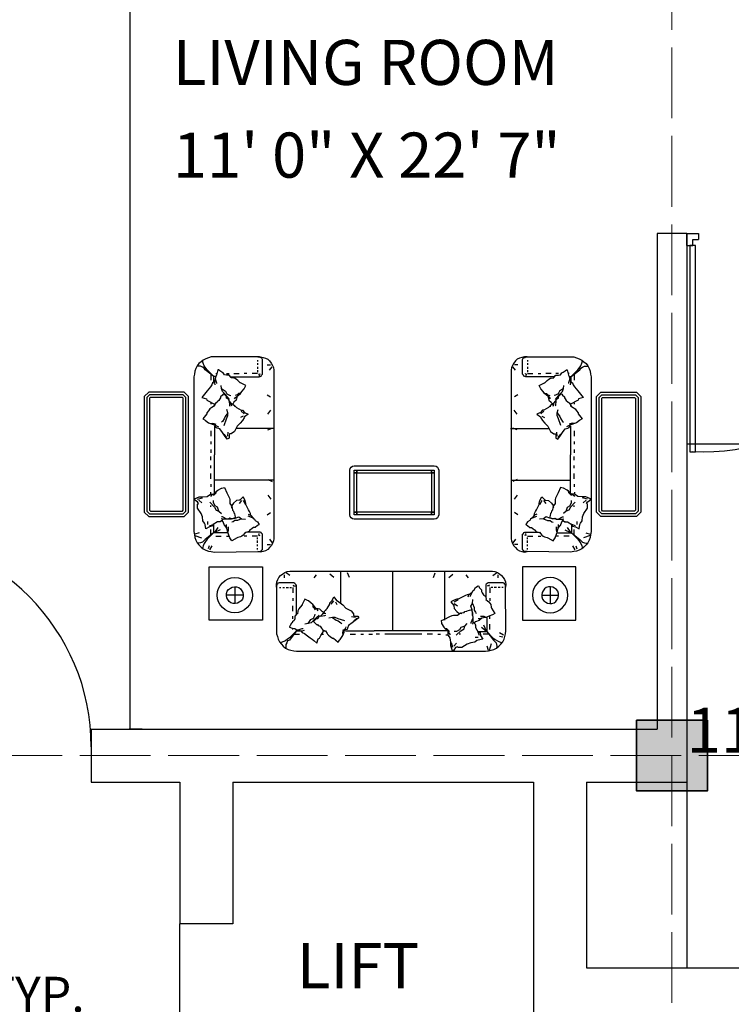
# Model space of a CAD drawing. Units: inches. Extents: x -113 to 5399, y -1393 to 3302.
# Tile 7 of 40: x 1073 to 1194, y 460 to 627. Entities that reach past the tile are written whole.
import ezdxf

# ---------------------------------------------------------------- set-up
doc = ezdxf.new("R2010")
doc.units = ezdxf.units.IN
doc.header["$MEASUREMENT"] = 0
doc.linetypes.add('ACAD_ISO02W100', pattern=[15, 12, -3])
doc.layers.add('24', color=7, linetype='Continuous')
for name, color, linetype, lineweight in [('A-ANNO-DIMS', 254, 'Continuous', 18), ('A-AREA-IDEN', 4, 'Continuous', 18), ('A-COLS', 7, 'Continuous', 35), ('doors', 2, 'Continuous', 25), ('furniture', 131, 'Continuous', 18), ('GRIDS', 7, 'ACAD_ISO02W100', 13), ('walls', 1, 'Continuous', 25)]:
    doc.layers.add(name, color=color, linetype=linetype, lineweight=lineweight)
doc.styles.get("Standard").update_dxf_attribs({"font": 'arial.ttf'})
doc.dimstyles.get("Standard").update_dxf_attribs({"dimtxt": 6, "dimasz": 0.18, "dimexe": 0.18, "dimexo": 0.0625, "dimgap": 0.09, "dimtad": 0, "dimtih": 1, "dimtoh": 1, "dimdec": 1, "dimzin": 0, "dimdsep": 46, "dimlunit": 4, "dimtxsty": 'Standard', "dimblk": 'ARCHTICK', "dimcen": 0.09, "dimadec": 0, "dimazin": 0, "dimtfac": 1, "dimtdec": 1, "dimtofl": 0, "dimtmove": 0, "dimatfit": 3, "dimfxl": 1, "dimtolj": 1, "dimtzin": 0, "dimarcsym": 0})

# ---------------------------------------------------------------- blocks, each defined once
blk = doc.blocks.new('*U3')
for p, q in [((0, 0), (0, -6)), ((36, 0), (36, -6))]:
    blk.add_line(p, q)
blk.add_lwpolyline([(0, 0), (0, 36), (1.75, 36), (1.75, 0)], close=True)
blk.add_arc((0, 0), 36, 0, 90)
blk = doc.blocks.new('DL13712')
at = {"layer": '24'}
for p, q in [((33, 28.5), (-34, 28.5)), ((33.5, -29.5), (-10, -29.5))]:
    blk.add_line(p, q, dxfattribs=at)
blk = doc.blocks.new('DL13976')
at = {"layer": '24'}
for p, q in [((-16, 11), (-13.5, 14)), ((-13.5, 14), (-10.5, 16.5)), ((-10.5, 16.5), (-7, 18.5)), ((-7, 18.5), (-3.5, 19.5)), ((-3.5, 19.5), (0.5, 20)), ((0.5, 20), (4.5, 19.5)), ((4.5, 19.5), (8, 18.5)), ((8, 18.5), (11.5, 16.5)), ((11.5, 16.5), (14.5, 14)), ((14.5, 14), (17, 11)), ((-19.5, 0), (-19, 4)), ((-19, -4), (-19.5, 0)), ((-19, 4), (-18, 7.5)), ((-18, 7.5), (-16, 11)), ((-9, 2), (-8, 4.5)), ((-9, -0.5), (-9, 2)), ((-9, 0), (10, 0)), ((-8, 4.5), (-6.5, 6.5)), ((-6.5, 6.5), (-4.5, 8)), ((-5.5, 0), (6.5, 0)), ((-4.5, 8), (-2.5, 9)), ((-2.5, 9), (0, 9.5)), ((0, 9.5), (2.5, 9.5)), ((0.5, -9.5), (0.5, 9.5)), ((0.5, -6), (0.5, 6)), ((2.5, 9.5), (5, 8.5)), ((5, 8.5), (7, 7)), ((7, 7), (8.5, 5)), ((8.5, 5), (9.5, 3)), ((9.5, 3), (10, 0.5)), ((10, 0.5), (10, -2)), ((17, 11), (19, 7.5)), ((19, 7.5), (20, 4)), ((20, 4), (20.5, 0)), ((20.5, 0), (20, -4)), ((-18, -7.5), (-19, -4)), ((-16, -11), (-18, -7.5)), ((-13.5, -14), (-16, -11)), ((-8.5, -3), (-9, -0.5)), ((-7.5, -5), (-8.5, -3)), ((-6, -7), (-7.5, -5)), ((-4, -8.5), (-6, -7)), ((-1.5, -9.5), (-4, -8.5)), ((1, -9.5), (-1.5, -9.5)), ((3.5, -9), (1, -9.5)), ((5.5, -8), (3.5, -9)), ((7.5, -6.5), (5.5, -8)), ((9, -4.5), (7.5, -6.5)), ((10, -2), (9, -4.5)), ((17, -11), (14.5, -14)), ((19, -7.5), (17, -11)), ((20, -4), (19, -7.5)), ((-10.5, -16.5), (-13.5, -14)), ((-7, -18.5), (-10.5, -16.5)), ((-3.5, -19.5), (-7, -18.5)), ((0.5, -20), (-3.5, -19.5)), ((4.5, -19.5), (0.5, -20)), ((8, -18.5), (4.5, -19.5)), ((11.5, -16.5), (8, -18.5)), ((14.5, -14), (11.5, -16.5))]:
    blk.add_line(p, q, dxfattribs=at)
blk = doc.blocks.new('DL13329')
at = {"layer": '24'}
for p, q in [((0, 0), (0, -60)), ((60, 0), (0, 0)), ((60, -60), (60, 0)), ((0, -60), (60, -60))]:
    blk.add_line(p, q, dxfattribs=at)
blk = doc.blocks.new('DL13303')
at = {"layer": '24'}
for p, q in [((-70, 20), (-65, 25)), ((-65, 25), (65, 25)), ((65, 25), (70, 20)), ((-70, -20), (-70, 20)), ((-67, 19), (-64, 22)), ((-67, -19), (-67, 19)), ((-64, 22), (64, 22)), ((-64, 18), (-63, 19)), ((-64, -18), (-64, 18)), ((-63, 19), (63, 19)), ((63, 19), (64, 18)), ((64, 22), (67, 19)), ((64, 18), (64, -18)), ((67, 19), (67, -19)), ((70, 20), (70, -20)), ((-65, -25), (-70, -20)), ((-64, -22), (-67, -19)), ((-63, -19), (-64, -18)), ((64, -22), (-64, -22)), ((63, -19), (-63, -19)), ((64, -18), (63, -19)), ((67, -19), (64, -22)), ((70, -20), (65, -25)), ((65, -25), (-65, -25))]:
    blk.add_line(p, q, dxfattribs=at)
blk = doc.blocks.new('DL12701')
at = {"layer": '24'}
for p, q in [((-96.5, 43.5), (-93.5, 44.5)), ((-93.5, 44.5), (-90, 45)), ((-90, 45), (-87, 45.5)), ((-87, 45.5), (0, 45.5)), ((0, 45.5), (87, 45.5)), ((50, 45), (48, 39.5)), ((51.5, 44.5), (50, 45)), ((53.5, 41.5), (51.5, 44.5)), ((87, 45.5), (90.5, 45)), ((88.5, 39.5), (90, 44.5)), ((90.5, 45), (93.5, 44.5)), ((91.5, 44.5), (94, 37)), ((93.5, 44.5), (96.5, 43.5)), ((-107.5, 32), (-106, 35)), ((-106, 35), (-104, 37.5)), ((-102.5, 35), (-105, 36)), ((-104, 37.5), (-102, 40)), ((-99.5, 34), (-102.5, 35)), ((-102, 40), (-99.5, 42)), ((-99.5, 42), (-96.5, 43.5)), ((-97, 32), (-99.5, 34)), ((-99, 40), (-99, 42)), ((-99, 38), (-99, 40)), ((-98, 36), (-99, 38)), ((-97, 34), (-98, 36)), ((-95, 33), (-97, 34)), ((-69.5, 32), (-67.5, 33.5)), ((-67.5, 33.5), (-64, 36.5)), ((-64, 36.5), (-62.5, 31.5)), ((-45.5, 31), (-40, 35.5)), ((-40, 35.5), (-38.5, 33)), ((48, 35.5), (47.5, 30.5)), ((48, 39.5), (48, 35.5)), ((50.5, 41.5), (49, 36)), ((51.5, 40), (54.5, 36.5)), ((55.5, 40.5), (53.5, 41.5)), ((56, 41.5), (55.5, 40.5)), ((60.5, 41.5), (56, 41.5)), ((66.5, 37.5), (60.5, 41.5)), ((70.5, 36), (66.5, 37.5)), ((75, 35.5), (70.5, 36)), ((77.5, 33.5), (75, 35.5)), ((79, 33), (77.5, 33.5)), ((96, 33), (97.5, 34.5)), ((96.5, 43.5), (99.5, 42)), ((97.5, 34.5), (99, 36)), ((98, 32.5), (100.5, 34)), ((99, 36), (99.5, 38)), ((99.5, 42), (102, 40)), ((100, 40), (99.5, 42)), ((99.5, 38), (100, 40)), ((100.5, 34), (103, 35)), ((102, 40), (104.5, 37.5)), ((103, 35), (106, 36)), ((104.5, 37.5), (106.5, 35)), ((106.5, 35), (108, 32)), ((-109.5, 26), (-108.5, 29)), ((-109.5, 22.5), (-109.5, 26)), ((-109.5, -26.5), (-109.5, 22.5)), ((-108.5, 29), (-107.5, 32)), ((-95, 30.5), (-97, 32)), ((-87.5, 23), (-95, 33)), ((-87.5, 23), (-95, 30.5)), ((-89.5, 26.5), (-83.5, 26.5)), ((-87.5, 21), (-87.5, 23)), ((-81.5, 23), (-87.5, 23)), ((-85, 21.5), (-82, 22.5)), ((-82, 22.5), (-80.5, 24.5)), ((-82, 22.5), (-80.5, 22.5)), ((-80.5, 24.5), (-78, 25.5)), ((-80.5, 24.5), (-80.5, 23.5)), ((-80.5, 22.5), (-78, 22)), ((-78, 25.5), (-76, 27)), ((-77, 25.5), (-77, 25.5)), ((-76, 27), (-71.5, 30.5)), ((-71.5, 30.5), (-69.5, 32)), ((-62.5, 31.5), (-61, 31)), ((-61, 31), (-59.5, 28)), ((-59.5, 28), (-57.5, 24.5)), ((-58, 26.5), (-56.5, 26.5)), ((-58, 21), (-54.5, 23)), ((-57.5, 24.5), (-56.5, 22)), ((-56.5, 22.5), (-54.5, 22.5)), ((-54.5, 22.5), (-52.5, 25.5)), ((-54.5, 23), (-54.5, 22.5)), ((-54, 22.5), (-54, 22.5)), ((-52.5, 25.5), (-52, 26.5)), ((-52, 26.5), (-51, 27.5)), ((-51, 27.5), (-49, 29)), ((-49, 29), (-46.5, 31)), ((-46.5, 31), (-45.5, 31)), ((-38.5, 33), (-38, 32.5)), ((-38, 32.5), (-35.5, 29)), ((-35.5, 29), (-34.5, 27)), ((-34.5, 27), (-35, 24.5)), ((-35, 24.5), (-34.5, 23)), ((-34.5, 27), (-33.5, 24)), ((-34.5, 23), (-34, 21)), ((-33.5, 24), (-33, 22)), ((-32, 22.5), (0.5, 22.5)), ((-26.5, 26.5), (-20.5, 26.5)), ((-14.5, 26.5), (-11.5, 26.5)), ((-5.5, 26.5), (-1.5, 26.5)), ((44, 22.5), (0.5, 22.5)), ((6.5, 26.5), (2.5, 26.5)), ((15.5, 26.5), (12.5, 26.5)), ((27.5, 26.5), (21.5, 26.5)), ((33.5, 26.5), (36.5, 26.5)), ((42.5, 27), (45, 27)), ((45, 23.5), (43.5, 22)), ((45.5, 28), (45, 27)), ((45, 27), (45, 23.5)), ((45, 23.5), (46.5, 26)), ((46.5, 23.5), (45, 22)), ((47.5, 30.5), (45.5, 28)), ((46.5, 26), (47.5, 27)), ((54.5, 23.5), (52, 23.5)), ((54, 27.5), (59.5, 22.5)), ((58, 21.5), (54.5, 23.5)), ((59, 26.5), (57.5, 26.5)), ((59.5, 22.5), (63, 20.5)), ((79, 30), (75.5, 30)), ((76, 19), (79, 24)), ((84, 32), (79, 33)), ((80.5, 28), (79, 24)), ((79, 24), (81, 24.5)), ((79, 23.5), (88.5, 23.5)), ((81, 24.5), (81.5, 28)), ((81.5, 28), (84, 32)), ((82.5, 18.5), (88, 22.5)), ((90.5, 26.5), (84.5, 26.5)), ((85, 16), (88, 22.5)), ((88.5, 23.5), (96, 33)), ((88.5, 23.5), (95.5, 30.5)), ((88.5, 8), (88.5, 23.5)), ((95.5, 30.5), (98, 32.5)), ((103, 28.5), (106.5, 29.5)), ((107.5, 27.5), (103, 25)), ((108, 32), (109, 29)), ((109, 29), (109.5, 26)), ((109.5, 26), (110, 22.5)), ((110, 22.5), (109.5, -26.5)), ((-95, 18.5), (-92, 19.5)), ((-95, 18), (-95, 18.5)), ((-94, 16.5), (-95, 18)), ((-92.5, 14), (-94, 16.5)), ((-92, 13.5), (-92.5, 14)), ((-92, 19.5), (-89, 20)), ((-91.5, 12.5), (-92, 13.5)), ((-89.5, 11), (-91.5, 12.5)), ((-91, 21), (-91, 19.5)), ((-89, 20), (-87.5, 21)), ((-87.5, 21), (-85, 21.5)), ((-85, 21.5), (-80.5, 20)), ((-80.5, 20), (-79.5, 20)), ((-74, 14.5), (-77.5, 15)), ((-70.5, 13.5), (-74, 14.5)), ((-74, 14.5), (-71, 10)), ((-67.5, 10.5), (-70.5, 13.5)), ((-68, 12), (-67.5, 12.5)), ((-65, 9), (-68, 12)), ((-67.5, 12.5), (-66.5, 13.5)), ((-66.5, 13.5), (-64.5, 15.5)), ((-64.5, 15.5), (-63.5, 15.5)), ((-63.5, 15.5), (-62.5, 16.5)), ((-62.5, 16.5), (-60.5, 17.5)), ((-60.5, 17.5), (-59, 19.5)), ((-59, 19.5), (-58.5, 19.5)), ((-58.5, 19.5), (-58, 21)), ((-42.5, 10.5), (-40, 11.5)), ((-40, 11.5), (-37, 13.5)), ((-32.5, 11.5), (-40, 9)), ((-37, 13.5), (-36, 14.5)), ((-30, 21), (-33, 22)), ((-33, 22), (-31.5, 19.5)), ((-31.5, 19.5), (-31, 18)), ((-29.5, 19.5), (-30, 21)), ((-28.5, 16.5), (-29.5, 19.5)), ((-24.5, 13.5), (-28.5, 16.5)), ((-21, 11), (-24.5, 13.5)), ((-19, 8.5), (-22.5, 11.5)), ((38, 14), (37.5, 11)), ((40.5, 18.5), (38, 14.5)), ((38, 14.5), (38, 14)), ((41.5, 20), (40.5, 18.5)), ((43.5, 22), (41.5, 20)), ((43.5, 20.5), (41.5, 20)), ((45, 22), (43.5, 20.5)), ((59.5, 19), (58, 21.5)), ((64, 17.5), (59.5, 19)), ((63, 20.5), (64, 17.5)), ((64, 17.5), (66.5, 14.5)), ((70.5, 13.5), (70.5, 14.5)), ((73, 8.5), (70.5, 13.5)), ((73, 13), (72.5, 15)), ((73, 12.5), (75, 14.5)), ((73, 12.5), (73, 13)), ((73, 8.5), (73, 12.5)), ((76, 12.5), (74, 14)), ((75, 14.5), (76, 16)), ((75.5, 16), (76, 16.5)), ((76, 16), (76, 19)), ((80, 11), (76, 12.5)), ((92, 21), (92, 15)), ((-91, 9), (-91, 6)), ((-91, 0.5), (-91, -5.5)), ((-89, 9), (-89.5, 11)), ((-89, 8.5), (-89, 9)), ((-89, 6), (-89, 8.5)), ((-86.5, 3.5), (-89, 6)), ((-87, 3.5), (-87, -26.5)), ((-86, 3.5), (-86.5, 3.5)), ((-85.5, 0.5), (-86, 3.5)), ((-85.5, 0), (-85.5, 0.5)), ((-84.5, -2), (-85.5, 0)), ((-71, 10), (-68, 8.5)), ((-68, 8.5), (-66.5, 5.5)), ((-61.5, 5.5), (-67.5, 10.5)), ((-66.5, 5.5), (-66, 4)), ((-63, 9), (-65, 9)), ((-62.5, 0), (-63.5, -1)), ((-62, 6.5), (-63, 9)), ((-60, 6), (-62, 6.5)), ((-61, -2), (-58.5, 0.5)), ((-57.5, 3.5), (-60, 6)), ((-60, 6), (-55, 5.5)), ((-58.5, 0.5), (-55.5, 2)), ((-56.5, 3.5), (-57.5, 3.5)), ((-57.5, 3.5), (-56, 1.5)), ((-54, 3), (-56.5, 3.5)), ((-56, 1.5), (-55, 0)), ((-55, 5.5), (-54, 5)), ((-55, 0), (-52.5, -2.5)), ((-46.5, 7.5), (-50.5, 8.5)), ((-46.5, 7.5), (-42.5, 10.5)), ((-43.5, 7.5), (-46.5, 7.5)), ((-40, 9), (-43.5, 7.5)), ((-31.5, -3), (-25.5, 0)), ((-25.5, 0), (-23, 3.5)), ((-20.5, 7.5), (-25, 7)), ((-23, 5.5), (-21.5, 6)), ((-23, 3.5), (-23, 5.5)), ((-21.5, 6), (-18, 6)), ((-17, 8), (-21, 11)), ((-18, 6), (-17, 8)), ((37.5, 11), (43.5, 8.5)), ((43.5, 8.5), (44, 8)), ((44, 8), (47, 6.5)), ((47, 6.5), (49.5, 5.5)), ((49.5, 5.5), (51, 5)), ((51, 5), (52.5, 5)), ((52, -2.5), (55, 1)), ((52.5, 5), (55.5, 5)), ((55, 1), (57.5, 3)), ((55.5, 5), (55.5, 5)), ((55.5, 5), (59, 2.5)), ((59, 2.5), (60, 3.5)), ((60, 3.5), (60, 2.5)), ((60, 2.5), (63, 2)), ((63, 2), (64, 1)), ((64, 1), (66, 0.5)), ((66, 0.5), (66.5, 0)), ((66.5, 0), (69, -0.5)), ((71.5, -1), (72.5, 2.5)), ((72, 5), (73, 6.5)), ((73, 5.5), (72, -1)), ((72.5, 2.5), (72, 5)), ((73, 6.5), (73, 8.5)), ((74.5, -0.5), (76, 1.5)), ((76, 1.5), (76.5, 3)), ((80.5, 9), (79, 9)), ((80.5, 10.5), (80, 11)), ((83, 8.5), (80.5, 10.5)), ((83, 8.5), (80.5, 9)), ((84, 6.5), (81.5, 6.5)), ((85, 8), (83, 8.5)), ((85.5, 6.5), (84, 6.5)), ((88, 7.5), (85, 8)), ((88, 7.5), (85.5, 6.5)), ((90, 6.5), (88, 7.5)), ((94, 5), (90, 6.5)), ((92, 9), (92, 6)), ((95, 4.5), (94, 5)), ((94, -3), (97.5, 3)), ((97.5, 3), (95, 4.5)), ((-91, -14), (-91, -11)), ((-83, -4), (-84.5, -2)), ((-80.5, -6.5), (-83, -4)), ((-80.5, -7), (-80.5, -6.5)), ((-77.5, -13), (-80.5, -7)), ((-73.5, -11), (-74.5, -11.5)), ((-70.5, -8.5), (-73.5, -11)), ((-68.5, -7), (-70.5, -8.5)), ((-68.5, -4.5), (-67, -3)), ((-66.5, -4.5), (-68.5, -7)), ((-68.5, -7), (-68.5, -4.5)), ((-67, -3), (-66, -1)), ((-65.5, -3), (-66.5, -4.5)), ((-63.5, -1), (-65.5, -3)), ((-65.5, -3), (-62.5, -2.5)), ((-62.5, -2.5), (-61, -2)), ((-54, -0.5), (-53.5, -0.5)), ((-52.5, -2.5), (-49.5, -7.5)), ((-49.5, -7.5), (-49.5, -9)), ((-49.5, -9), (-47, -11.5)), ((-45.5, -11), (-48.5, -7.5)), ((-43, -10), (-41.5, -7)), ((-42, -11.5), (-41, -11)), ((-41, -11), (-38, -9)), ((-38, -9), (-35, -6.5)), ((-35, -6.5), (-31.5, -3)), ((48, -10), (51.5, -6)), ((52, -12), (48, -10)), ((51.5, -5.5), (52, -2.5)), ((51.5, -6), (51.5, -5.5)), ((52, -8), (55.5, -5.5)), ((52, -10), (56.5, -12.5)), ((69, -0.5), (70.5, -1)), ((70.5, -1), (71.5, -1)), ((72, -1), (70.5, -5)), ((70.5, -5), (72.5, -8)), ((72.5, -8), (74.5, -3.5)), ((72.5, -8), (73, -12.5)), ((74.5, -3.5), (74.5, -0.5)), ((87.5, -12.5), (89.5, -11)), ((89.5, -11), (91, -10)), ((91, -10), (92, -8.5)), ((92, -8.5), (93, -7)), ((92, -14), (92, -11)), ((93, -7), (93.5, -4)), ((93.5, -4), (94, -3)), ((-91, -26), (-91, -20)), ((-74.5, -11.5), (-77.5, -13)), ((-47, -11.5), (-45, -15.5)), ((-45, -15.5), (-42, -11.5)), ((55, -13), (52, -12)), ((56.5, -13), (55, -13)), ((62.5, -16), (56.5, -13)), ((64.5, -17), (62.5, -16)), ((64, -16.5), (64, -16.5)), ((66.5, -18), (64.5, -17)), ((69, -18.5), (66.5, -18)), ((67.5, -15.5), (68.5, -18)), ((68.5, -18), (69, -18.5)), ((69, -18.5), (72, -21)), ((70, -16.5), (69.5, -15.5)), ((72, -21), (70, -16.5)), ((72, -21), (73, -22.5)), ((82.5, -21.5), (83.5, -20)), ((82.5, -22.5), (82.5, -21.5)), ((83.5, -20), (85, -18)), ((85, -17.5), (87, -16.5)), ((85, -18), (85, -17.5)), ((87, -16.5), (88, -13)), ((88, -13), (87.5, -12.5)), ((87.5, -26.5), (87.5, -14.5)), ((92, -26), (92, -20)), ((-109.5, -28), (-109.5, -26.5)), ((-109.5, -26.5), (-109.5, -29.5)), ((-109, -29), (-109.5, -28)), ((-109.5, -29.5), (-109, -32.5)), ((-108.5, -30), (-109, -29)), ((-109, -32.5), (-108, -35)), ((-108, -31), (-108.5, -30)), ((-106.5, -31.5), (-108, -31)), ((-105.5, -31.5), (-106.5, -31.5)), ((-106, -26), (-104.5, -26)), ((-104.5, -31.5), (-105.5, -31.5)), ((-92, -31.5), (-104.5, -31.5)), ((-102.5, -26), (-100.5, -26)), ((-98.5, -26), (-96, -26)), ((-94.5, -26), (-92.5, -26)), ((-91, -31.5), (-92, -31.5)), ((-90, -31.5), (-91, -31.5)), ((-90.5, -27.5), (-88, -28)), ((-90.5, -28), (-90, -29)), ((-89, -30.5), (-90, -31.5)), ((-88, -30), (-89, -30.5)), ((-87.5, -29), (-88, -30)), ((-87, -28), (-87.5, -29)), ((-87, -26.5), (-87, -28)), ((73, -22.5), (74.5, -23.5)), ((74.5, -23.5), (76, -26)), ((76, -26), (79, -28)), ((79, -28), (79.5, -27.5)), ((79.5, -27.5), (80, -26)), ((80, -26), (82.5, -23.5)), ((82.5, -23.5), (82.5, -22.5)), ((87.5, -28), (87.5, -26.5)), ((87.5, -29), (87.5, -28)), ((88, -30), (87.5, -29)), ((89, -30.5), (88, -30)), ((91.5, -27.5), (89, -28)), ((90, -31.5), (89, -30.5)), ((91, -31.5), (90, -31.5)), ((91.5, -28), (91, -29)), ((92.5, -31.5), (91, -31.5)), ((104.5, -31.5), (92.5, -31.5)), ((95.5, -26), (93.5, -26)), ((99.5, -26), (97, -26)), ((103.5, -26), (101.5, -26)), ((106, -31.5), (104.5, -31.5)), ((107, -26), (105.5, -26)), ((107, -31.5), (106, -31.5)), ((108, -31), (107, -31.5)), ((109, -30), (108, -31)), ((108.5, -35), (109.5, -32.5)), ((109.5, -29), (109, -30)), ((110, -29.5), (109.5, -26.5)), ((109.5, -26.5), (109.5, -28)), ((109.5, -28), (109.5, -29)), ((109.5, -32.5), (110, -29.5)), ((-108, -35), (-107, -37.5)), ((-107, -37.5), (-105, -39.5)), ((-105, -39.5), (-102.5, -41.5)), ((-102.5, -41.5), (-100, -43)), ((-100.5, -37), (-100.5, -40.5)), ((-100, -43), (-97.5, -44)), ((-94.5, -39.5), (-98.5, -42.5)), ((-97.5, -44), (-94.5, -44.5)), ((-67, -37), (-64.5, -40.5)), ((-45, -37.5), (-49.5, -41)), ((-27.5, -37.5), (-29.5, -42.5)), ((28.5, -37.5), (30.5, -42.5)), ((46, -37.5), (50.5, -41)), ((68, -37), (65.5, -40.5)), ((95, -44.5), (97.5, -44)), ((95.5, -39.5), (99.5, -42.5)), ((97.5, -44), (100.5, -43)), ((100.5, -43), (103, -41.5)), ((101.5, -37), (101.5, -40.5)), ((103, -41.5), (105, -39.5)), ((105, -39.5), (107, -37.5)), ((107, -37.5), (108.5, -35)), ((-94.5, -44.5), (0, -44.5)), ((0, -44.5), (95, -44.5))]:
    blk.add_line(p, q, dxfattribs=at)
blk = doc.blocks.new('DL13707')
at = {"layer": '24'}
for p, q in [((0, -33.5), (0, 33.5)), ((-58.5, -33.5), (-58.5, 21.5)), ((58.5, -33.5), (58.5, 2))]:
    blk.add_line(p, q, dxfattribs=at)
blk = doc.blocks.new('DL13651')
at = {"layer": '24'}
for p, q in [((-50.5, 25), (-50, 27)), ((-50.5, -25), (-50.5, 25)), ((-50, 27), (-49, 28.5)), ((-49, 28.5), (-47.5, 29.5)), ((-47.5, 29.5), (-45.5, 30)), ((-45.5, 30), (44.5, 30)), ((-45.5, 24.5), (-45.5, 25)), ((-45.5, 25), (-45, 25)), ((-45.5, -24.5), (-45.5, 24.5)), ((-45, 25), (44, 25)), ((-42.5, -24.5), (-42.5, 24.5)), ((-42.5, 24.5), (-42.5, 22)), ((41.5, 22), (41.5, 24.5)), ((41.5, 24.5), (41.5, -24.5)), ((44, 25), (44.5, 25)), ((44.5, 30), (46.5, 29.5)), ((44.5, 25), (44.5, 24.5)), ((44.5, 24.5), (44.5, -24.5)), ((46.5, 29.5), (48, 28.5)), ((48, 28.5), (49, 27)), ((49, 27), (49.5, 25)), ((49.5, 25), (49.5, -25)), ((-45, 22), (44, 22)), ((-42.5, 22), (-45, 22)), ((44, 22), (41.5, 22)), ((44, -22), (-45, -22)), ((-45, -22), (-42.5, -22)), ((-42.5, -22), (-42.5, -24.5)), ((41.5, -24.5), (41.5, -22)), ((41.5, -22), (44, -22)), ((-50, -27), (-50.5, -25)), ((-49, -28.5), (-50, -27)), ((-47.5, -29.5), (-49, -28.5)), ((-45.5, -30), (-47.5, -29.5)), ((-45.5, -25), (-45.5, -24.5)), ((-45, -25), (-45.5, -25)), ((44.5, -30), (-45.5, -30)), ((44, -25), (-45, -25)), ((44.5, -25), (44, -25)), ((44.5, -24.5), (44.5, -25)), ((46.5, -29.5), (44.5, -30)), ((48, -28.5), (46.5, -29.5)), ((49, -27), (48, -28.5)), ((49.5, -25), (49, -27))]:
    blk.add_line(p, q, dxfattribs=at)
blk = doc.blocks.new('DL12263')
at = {"layer": '24'}
for p, q in [((-115.5, 43.5), (-112.5, 44.5)), ((-112.5, 44.5), (-109, 45)), ((-109, 45), (-106, 45.5)), ((-106, 45.5), (-19, 45.5)), ((-19, 45.5), (106.5, 45.5)), ((69.5, 45), (67.5, 39.5)), ((71, 44.5), (69.5, 45)), ((73, 41.5), (71, 44.5)), ((106.5, 45.5), (110, 45)), ((108, 39.5), (109.5, 44.5)), ((110, 45), (113, 44.5)), ((111, 44.5), (113.5, 37)), ((113, 44.5), (116, 43.5)), ((-126.5, 32), (-125, 35)), ((-125, 35), (-123, 37.5)), ((-121.5, 35), (-124, 36)), ((-123, 37.5), (-121, 40)), ((-118.5, 34), (-121.5, 35)), ((-121, 40), (-118.5, 42)), ((-118.5, 42), (-115.5, 43.5)), ((-116, 32), (-118.5, 34)), ((-118, 40), (-118, 42)), ((-118, 38), (-118, 40)), ((-117, 36), (-118, 38)), ((-116, 34), (-117, 36)), ((-114, 33), (-116, 34)), ((-88.5, 32), (-86.5, 33.5)), ((-86.5, 33.5), (-83, 36.5)), ((-83, 36.5), (-81.5, 31.5)), ((-64.5, 31), (-59, 35.5)), ((-59, 35.5), (-57.5, 33)), ((67.5, 35.5), (67, 30.5)), ((67.5, 39.5), (67.5, 35.5)), ((70, 41.5), (68.5, 36)), ((71, 40), (74, 36.5)), ((75, 40.5), (73, 41.5)), ((75.5, 41.5), (75, 40.5)), ((80, 41.5), (75.5, 41.5)), ((86, 37.5), (80, 41.5)), ((90, 36), (86, 37.5)), ((94.5, 35.5), (90, 36)), ((97, 33.5), (94.5, 35.5)), ((98.5, 33), (97, 33.5)), ((115.5, 33), (117, 34.5)), ((116, 43.5), (119, 42)), ((117, 34.5), (118.5, 36)), ((117.5, 32.5), (120, 34)), ((118.5, 36), (119, 38)), ((119, 42), (121.5, 40)), ((119.5, 40), (119, 42)), ((119, 38), (119.5, 40)), ((120, 34), (122.5, 35)), ((121.5, 40), (124, 37.5)), ((122.5, 35), (125.5, 36)), ((124, 37.5), (126, 35)), ((126, 35), (127.5, 32)), ((-128.5, 26), (-127.5, 29)), ((-128.5, 22.5), (-128.5, 26)), ((-128.5, -26.5), (-128.5, 22.5)), ((-127.5, 29), (-126.5, 32)), ((-114, 30.5), (-116, 32)), ((-106.5, 23), (-114, 33)), ((-106.5, 23), (-114, 30.5)), ((-108.5, 26.5), (-102.5, 26.5)), ((-106.5, 21), (-106.5, 23)), ((-100.5, 23), (-106.5, 23)), ((-104, 21.5), (-101, 22.5)), ((-101, 22.5), (-99.5, 24.5)), ((-101, 22.5), (-99.5, 22.5)), ((-99.5, 24.5), (-97, 25.5)), ((-99.5, 24.5), (-99.5, 23.5)), ((-99.5, 22.5), (-97, 22)), ((-97, 25.5), (-95, 27)), ((-96, 25.5), (-96, 25.5)), ((-95, 27), (-90.5, 30.5)), ((-90.5, 30.5), (-88.5, 32)), ((-81.5, 31.5), (-80, 31)), ((-80, 31), (-78.5, 28)), ((-78.5, 28), (-76.5, 24.5)), ((-77, 26.5), (-75.5, 26.5)), ((-77, 21), (-73.5, 23)), ((-76.5, 24.5), (-75.5, 22)), ((-75.5, 22.5), (-73.5, 22.5)), ((-73.5, 22.5), (-71.5, 25.5)), ((-73.5, 23), (-73.5, 22.5)), ((-73, 22.5), (-73, 22.5)), ((-71.5, 25.5), (-71, 26.5)), ((-71, 26.5), (-70, 27.5)), ((-70, 27.5), (-68, 29)), ((-68, 29), (-65.5, 31)), ((-65.5, 31), (-64.5, 31)), ((-57.5, 33), (-57, 32.5)), ((-57, 32.5), (-54.5, 29)), ((-54.5, 29), (-53.5, 27)), ((-53.5, 27), (-54, 24.5)), ((-54, 24.5), (-53.5, 23)), ((-53.5, 27), (-52.5, 24)), ((-53.5, 23), (-53, 21)), ((-52.5, 24), (-52, 22)), ((-51, 22.5), (-18.5, 22.5)), ((-45.5, 26.5), (-39.5, 26.5)), ((-33.5, 26.5), (-30.5, 26.5)), ((-24.5, 26.5), (-20.5, 26.5)), ((63.5, 22.5), (-18.5, 22.5)), ((-12.5, 26.5), (-16.5, 26.5)), ((35, 26.5), (-6.5, 26.5)), ((47, 26.5), (41, 26.5)), ((53, 26.5), (56, 26.5)), ((62, 27), (64.5, 27)), ((64.5, 23.5), (63, 22)), ((65, 28), (64.5, 27)), ((64.5, 27), (64.5, 23.5)), ((64.5, 23.5), (66, 26)), ((66, 23.5), (64.5, 22)), ((67, 30.5), (65, 28)), ((66, 26), (67, 27)), ((74, 23.5), (71.5, 23.5)), ((73.5, 27.5), (79, 22.5)), ((77.5, 21.5), (74, 23.5)), ((78.5, 26.5), (77, 26.5)), ((79, 22.5), (82.5, 20.5)), ((98.5, 30), (95, 30)), ((95.5, 19), (98.5, 24)), ((103.5, 32), (98.5, 33)), ((100, 28), (98.5, 24)), ((98.5, 24), (100.5, 24.5)), ((98.5, 23.5), (108, 23.5)), ((100.5, 24.5), (101, 28)), ((101, 28), (103.5, 32)), ((102, 18.5), (107.5, 22.5)), ((110, 26.5), (104, 26.5)), ((104.5, 16), (107.5, 22.5)), ((108, 23.5), (115.5, 33)), ((108, 23.5), (115, 30.5)), ((108, 8), (108, 23.5)), ((115, 30.5), (117.5, 32.5)), ((122.5, 28.5), (126, 29.5)), ((127, 27.5), (122.5, 25)), ((127.5, 32), (128.5, 29)), ((128.5, 29), (129, 26)), ((129, 26), (129.5, 22.5)), ((129.5, 22.5), (129, -26.5)), ((-114, 18.5), (-111, 19.5)), ((-114, 18), (-114, 18.5)), ((-113, 16.5), (-114, 18)), ((-111.5, 14), (-113, 16.5)), ((-111, 13.5), (-111.5, 14)), ((-111, 19.5), (-108, 20)), ((-110.5, 12.5), (-111, 13.5)), ((-108.5, 11), (-110.5, 12.5)), ((-110, 21), (-110, 19.5)), ((-108, 20), (-106.5, 21)), ((-106.5, 21), (-104, 21.5)), ((-104, 21.5), (-99.5, 20)), ((-99.5, 20), (-98.5, 20)), ((-93, 14.5), (-96.5, 15)), ((-89.5, 13.5), (-93, 14.5)), ((-93, 14.5), (-90, 10)), ((-86.5, 10.5), (-89.5, 13.5)), ((-87, 12), (-86.5, 12.5)), ((-84, 9), (-87, 12)), ((-86.5, 12.5), (-85.5, 13.5)), ((-85.5, 13.5), (-83.5, 15.5)), ((-83.5, 15.5), (-82.5, 15.5)), ((-82.5, 15.5), (-81.5, 16.5)), ((-81.5, 16.5), (-79.5, 17.5)), ((-79.5, 17.5), (-78, 19.5)), ((-78, 19.5), (-77.5, 19.5)), ((-77.5, 19.5), (-77, 21)), ((-61.5, 10.5), (-59, 11.5)), ((-59, 11.5), (-56, 13.5)), ((-51.5, 11.5), (-59, 9)), ((-56, 13.5), (-55, 14.5)), ((-49, 21), (-52, 22)), ((-52, 22), (-50.5, 19.5)), ((-50.5, 19.5), (-50, 18)), ((-48.5, 19.5), (-49, 21)), ((-47.5, 16.5), (-48.5, 19.5)), ((-43.5, 13.5), (-47.5, 16.5)), ((-40, 11), (-43.5, 13.5)), ((-38, 8.5), (-41.5, 11.5)), ((57.5, 14), (57, 11)), ((60, 18.5), (57.5, 14.5)), ((57.5, 14.5), (57.5, 14)), ((61, 20), (60, 18.5)), ((63, 22), (61, 20)), ((63, 20.5), (61, 20)), ((64.5, 22), (63, 20.5)), ((79, 19), (77.5, 21.5)), ((83.5, 17.5), (79, 19)), ((82.5, 20.5), (83.5, 17.5)), ((83.5, 17.5), (86, 14.5)), ((90, 13.5), (90, 14.5)), ((92.5, 8.5), (90, 13.5)), ((92.5, 13), (92, 15)), ((92.5, 12.5), (94.5, 14.5)), ((92.5, 12.5), (92.5, 13)), ((92.5, 8.5), (92.5, 12.5)), ((95.5, 12.5), (93.5, 14)), ((94.5, 14.5), (95.5, 16)), ((95, 16), (95.5, 16.5)), ((95.5, 16), (95.5, 19)), ((99.5, 11), (95.5, 12.5)), ((111.5, 21), (111.5, 15)), ((-110, 9), (-110, 6)), ((-110, 0.5), (-110, -5.5)), ((-108, 9), (-108.5, 11)), ((-108, 8.5), (-108, 9)), ((-108, 6), (-108, 8.5)), ((-105.5, 3.5), (-108, 6)), ((-106, 3.5), (-106, -26.5)), ((-105, 3.5), (-105.5, 3.5)), ((-104.5, 0.5), (-105, 3.5)), ((-104.5, 0), (-104.5, 0.5)), ((-103.5, -2), (-104.5, 0)), ((-90, 10), (-87, 8.5)), ((-87, 8.5), (-85.5, 5.5)), ((-80.5, 5.5), (-86.5, 10.5)), ((-85.5, 5.5), (-85, 4)), ((-82, 9), (-84, 9)), ((-81.5, 0), (-82.5, -1)), ((-81, 6.5), (-82, 9)), ((-79, 6), (-81, 6.5)), ((-80, -2), (-77.5, 0.5)), ((-76.5, 3.5), (-79, 6)), ((-79, 6), (-74, 5.5)), ((-77.5, 0.5), (-74.5, 2)), ((-75.5, 3.5), (-76.5, 3.5)), ((-76.5, 3.5), (-75, 1.5)), ((-73, 3), (-75.5, 3.5)), ((-75, 1.5), (-74, 0)), ((-74, 5.5), (-73, 5)), ((-74, 0), (-71.5, -2.5)), ((-65.5, 7.5), (-69.5, 8.5)), ((-65.5, 7.5), (-61.5, 10.5)), ((-62.5, 7.5), (-65.5, 7.5)), ((-59, 9), (-62.5, 7.5)), ((-50.5, -3), (-44.5, 0)), ((-44.5, 0), (-42, 3.5)), ((-39.5, 7.5), (-44, 7)), ((-42, 5.5), (-40.5, 6)), ((-42, 3.5), (-42, 5.5)), ((-40.5, 6), (-37, 6)), ((-36, 8), (-40, 11)), ((-37, 6), (-36, 8)), ((57, 11), (63, 8.5)), ((63, 8.5), (63.5, 8)), ((63.5, 8), (66.5, 6.5)), ((66.5, 6.5), (69, 5.5)), ((69, 5.5), (70.5, 5)), ((70.5, 5), (72, 5)), ((71.5, -2.5), (74.5, 1)), ((72, 5), (75, 5)), ((74.5, 1), (77, 3)), ((75, 5), (75, 5)), ((75, 5), (78.5, 2.5)), ((78.5, 2.5), (79.5, 3.5)), ((79.5, 3.5), (79.5, 2.5)), ((79.5, 2.5), (82.5, 2)), ((82.5, 2), (83.5, 1)), ((83.5, 1), (85.5, 0.5)), ((85.5, 0.5), (86, 0)), ((86, 0), (88.5, -0.5)), ((91, -1), (92, 2.5)), ((91.5, 5), (92.5, 6.5)), ((92.5, 5.5), (91.5, -1)), ((92, 2.5), (91.5, 5)), ((92.5, 6.5), (92.5, 8.5)), ((94, -0.5), (95.5, 1.5)), ((95.5, 1.5), (96, 3)), ((100, 9), (98.5, 9)), ((100, 10.5), (99.5, 11)), ((102.5, 8.5), (100, 10.5)), ((102.5, 8.5), (100, 9)), ((103.5, 6.5), (101, 6.5)), ((104.5, 8), (102.5, 8.5)), ((105, 6.5), (103.5, 6.5)), ((107.5, 7.5), (104.5, 8)), ((107.5, 7.5), (105, 6.5)), ((109.5, 6.5), (107.5, 7.5)), ((113.5, 5), (109.5, 6.5)), ((111.5, 9), (111.5, 6)), ((114.5, 4.5), (113.5, 5)), ((113.5, -3), (117, 3)), ((117, 3), (114.5, 4.5)), ((-110, -14), (-110, -11)), ((-102, -4), (-103.5, -2)), ((-99.5, -6.5), (-102, -4)), ((-99.5, -7), (-99.5, -6.5)), ((-96.5, -13), (-99.5, -7)), ((-92.5, -11), (-93.5, -11.5)), ((-89.5, -8.5), (-92.5, -11)), ((-87.5, -7), (-89.5, -8.5)), ((-87.5, -4.5), (-86, -3)), ((-85.5, -4.5), (-87.5, -7)), ((-87.5, -7), (-87.5, -4.5)), ((-86, -3), (-85, -1)), ((-84.5, -3), (-85.5, -4.5)), ((-82.5, -1), (-84.5, -3)), ((-84.5, -3), (-81.5, -2.5)), ((-81.5, -2.5), (-80, -2)), ((-73, -0.5), (-72.5, -0.5)), ((-71.5, -2.5), (-68.5, -7.5)), ((-68.5, -7.5), (-68.5, -9)), ((-68.5, -9), (-66, -11.5)), ((-64.5, -11), (-67.5, -7.5)), ((-62, -10), (-60.5, -7)), ((-61, -11.5), (-60, -11)), ((-60, -11), (-57, -9)), ((-57, -9), (-54, -6.5)), ((-54, -6.5), (-50.5, -3)), ((67.5, -10), (71, -6)), ((71.5, -12), (67.5, -10)), ((71, -5.5), (71.5, -2.5)), ((71, -6), (71, -5.5)), ((71.5, -8), (75, -5.5)), ((71.5, -10), (76, -12.5)), ((88.5, -0.5), (90, -1)), ((90, -1), (91, -1)), ((91.5, -1), (90, -5)), ((90, -5), (92, -8)), ((92, -8), (94, -3.5)), ((92, -8), (92.5, -12.5)), ((94, -3.5), (94, -0.5)), ((107, -12.5), (109, -11)), ((109, -11), (110.5, -10)), ((110.5, -10), (111.5, -8.5)), ((111.5, -8.5), (112.5, -7)), ((111.5, -14), (111.5, -11)), ((112.5, -7), (113, -4)), ((113, -4), (113.5, -3)), ((-110, -26), (-110, -20)), ((-93.5, -11.5), (-96.5, -13)), ((-66, -11.5), (-64, -15.5)), ((-64, -15.5), (-61, -11.5)), ((74.5, -13), (71.5, -12)), ((76, -13), (74.5, -13)), ((82, -16), (76, -13)), ((84, -17), (82, -16)), ((83.5, -16.5), (83.5, -16.5)), ((86, -18), (84, -17)), ((88.5, -18.5), (86, -18)), ((87, -15.5), (88, -18)), ((88, -18), (88.5, -18.5)), ((88.5, -18.5), (91.5, -21)), ((89.5, -16.5), (89, -15.5)), ((91.5, -21), (89.5, -16.5)), ((91.5, -21), (92.5, -22.5)), ((102, -21.5), (103, -20)), ((102, -22.5), (102, -21.5)), ((103, -20), (104.5, -18)), ((104.5, -17.5), (106.5, -16.5)), ((104.5, -18), (104.5, -17.5)), ((106.5, -16.5), (107.5, -13)), ((107.5, -13), (107, -12.5)), ((107, -26.5), (107, -14.5)), ((111.5, -26), (111.5, -20)), ((-128.5, -28), (-128.5, -26.5)), ((-128.5, -26.5), (-128.5, -29.5)), ((-128, -29), (-128.5, -28)), ((-128.5, -29.5), (-128, -32.5)), ((-127.5, -30), (-128, -29)), ((-128, -32.5), (-127, -35)), ((-127, -31), (-127.5, -30)), ((-125.5, -31.5), (-127, -31)), ((-124.5, -31.5), (-125.5, -31.5)), ((-125, -26), (-123.5, -26)), ((-123.5, -31.5), (-124.5, -31.5)), ((-111, -31.5), (-123.5, -31.5)), ((-121.5, -26), (-119.5, -26)), ((-117.5, -26), (-115, -26)), ((-113.5, -26), (-111.5, -26)), ((-110, -31.5), (-111, -31.5)), ((-109, -31.5), (-110, -31.5)), ((-109.5, -27.5), (-107, -28)), ((-109.5, -28), (-109, -29)), ((-108, -30.5), (-109, -31.5)), ((-107, -30), (-108, -30.5)), ((-106.5, -29), (-107, -30)), ((-106, -28), (-106.5, -29)), ((-106, -26.5), (-106, -28)), ((92.5, -22.5), (94, -23.5)), ((94, -23.5), (95.5, -26)), ((95.5, -26), (98.5, -28)), ((98.5, -28), (99, -27.5)), ((99, -27.5), (99.5, -26)), ((99.5, -26), (102, -23.5)), ((102, -23.5), (102, -22.5)), ((107, -28), (107, -26.5)), ((107, -29), (107, -28)), ((107.5, -30), (107, -29)), ((108.5, -30.5), (107.5, -30)), ((111, -27.5), (108.5, -28)), ((109.5, -31.5), (108.5, -30.5)), ((110.5, -31.5), (109.5, -31.5)), ((111, -28), (110.5, -29)), ((112, -31.5), (110.5, -31.5)), ((124, -31.5), (112, -31.5)), ((115, -26), (113, -26)), ((119, -26), (116.5, -26)), ((123, -26), (121, -26)), ((125.5, -31.5), (124, -31.5)), ((126.5, -26), (125, -26)), ((126.5, -31.5), (125.5, -31.5)), ((127.5, -31), (126.5, -31.5)), ((128.5, -30), (127.5, -31)), ((128, -35), (129, -32.5)), ((129, -29), (128.5, -30)), ((129.5, -29.5), (129, -26.5)), ((129, -26.5), (129, -28)), ((129, -28), (129, -29)), ((129, -32.5), (129.5, -29.5)), ((-127, -35), (-126, -37.5)), ((-126, -37.5), (-124, -39.5)), ((-124, -39.5), (-121.5, -41.5)), ((-121.5, -41.5), (-119, -43)), ((-119.5, -37), (-119.5, -40.5)), ((-119, -43), (-116.5, -44)), ((-113.5, -39.5), (-117.5, -42.5)), ((-116.5, -44), (-113.5, -44.5)), ((-86, -37), (-83.5, -40.5)), ((-64, -37.5), (-68.5, -41)), ((-46.5, -37.5), (-48.5, -42.5)), ((48, -37.5), (50, -42.5)), ((65.5, -37.5), (70, -41)), ((87.5, -37), (85, -40.5)), ((114.5, -44.5), (117, -44)), ((115, -39.5), (119, -42.5)), ((117, -44), (120, -43)), ((120, -43), (122.5, -41.5)), ((121, -37), (121, -40.5)), ((122.5, -41.5), (124.5, -39.5)), ((124.5, -39.5), (126.5, -37.5)), ((126.5, -37.5), (128, -35)), ((-113.5, -44.5), (-19, -44.5)), ((-19, -44.5), (114.5, -44.5))]:
    blk.add_line(p, q, dxfattribs=at)
blk = doc.blocks.new('U3M')
at = {"yscale": 10, "zscale": 10}
for name, p, xscale, rotation in [('DL13303', (1315, 2544), -10, 180), ('DL13712', (1310, 1664), -10, 90), ('DL13976', (-270, 1769), 10, 90), ('DL12263', (-445, 20), -10, 90), ('DL13707', (-335, 0), 10, 90), ('DL13651', (885, -25), 10, 270), ('DL13712', (1310, -1664), 10, 90), ('DL12701', (1315, -1779), 10, 180), ('DL13329', (50, -2064), 10, 180), ('DL13976', (-270, -1769), -10, 90)]:
    blk.add_blockref(name, p, dxfattribs=dict(at, xscale=xscale, rotation=rotation))
for name, p, xscale in [('DL12701', (1315, 1779), -10), ('DL13329', (50, 2064), -10), ('DL13303', (1315, -2544), 10)]:
    blk.add_blockref(name, p, dxfattribs=dict(at, xscale=xscale))
at = {"flags": 3}
for tag in ['AECLAY', 'AECGTYPE']:
    blk.add_attdef(tag, (0, 0), '', height=0.5, dxfattribs=at)
blk = doc.blocks.new('_ArchTick')
at = {"color": 0, "linetype": 'ByBlock', "const_width": 0.15}
blk.add_lwpolyline([(-0.5, -0.5), (0.5, 0.5)], dxfattribs=at)
blk = doc.blocks.new('*D25')
at = {"layer": 'A-ANNO-DIMS', "color": 0, "lineweight": -2, "transparency": 16777216}
for p, q in [((1091.29, 777.53), (1092, 777.53)), ((1091.82, 777.53), (1091.82, 645.13)), ((1091.82, 506.53), (1091.82, 638.93)), ((1093.84, 506.53), (1091.64, 506.53))]:
    blk.add_line(p, q, dxfattribs=at)
at = {"layer": 'Defpoints', "color": 0, "transparency": 16777216}
for p in [(1091.23, 777.53), (1091.82, 777.53), (1093.91, 506.53)]:
    blk.add_point(p, dxfattribs=at)
at = {"layer": 'A-ANNO-DIMS', "color": 0, "lineweight": -2, "transparency": 16777216, "xscale": 0.18, "yscale": 0.18, "zscale": 0.18}
for p, rotation in [((1091.82, 777.53), 90), ((1091.82, 506.53), 270)]:
    blk.add_blockref('_ArchTick', p, dxfattribs=dict(at, rotation=rotation))
at = {"layer": 'A-ANNO-DIMS', "color": 0, "transparency": 16777216, "insert": (1091.82, 642.03), "char_height": 6, "attachment_point": 5}
blk.add_mtext('\\A1;22\'-7"', dxfattribs=at)
blk = doc.blocks.new('*D46')
at = {"layer": 'A-ANNO-DIMS', "color": 0, "lineweight": -2, "transparency": 16777216}
for p, q in [((1186.23, 554.92), (1186.23, 554.73)), ((1186.23, 554.91), (1247.33, 554.91)), ((1318.23, 554.91), (1257.13, 554.91)), ((1318.23, 554.92), (1318.23, 554.73))]:
    blk.add_line(p, q, dxfattribs=at)
at = {"layer": 'Defpoints', "color": 0, "transparency": 16777216}
for p in [(1186.23, 554.98), (1186.23, 554.91), (1318.23, 554.98)]:
    blk.add_point(p, dxfattribs=at)
at = {"layer": 'A-ANNO-DIMS', "color": 0, "lineweight": -2, "transparency": 16777216, "xscale": 0.18, "yscale": 0.18, "zscale": 0.18, "rotation": 180}
blk.add_blockref('_ArchTick', (1186.23, 554.91), dxfattribs=at)
at = {"layer": 'A-ANNO-DIMS', "color": 0, "lineweight": -2, "transparency": 16777216, "xscale": 0.18, "yscale": 0.18, "zscale": 0.18}
blk.add_blockref('_ArchTick', (1318.23, 554.91), dxfattribs=at)
at = {"layer": 'A-ANNO-DIMS', "color": 0, "transparency": 16777216, "insert": (1252.23, 554.91), "char_height": 6, "attachment_point": 5}
blk.add_mtext("\\A1;11'", dxfattribs=at)
blk = doc.blocks.new('COLUMN-12IN-SQUARE')
h = blk.add_hatch(color=256)
h.dxf.hatch_style = 1
h.paths.add_polyline_path([(6, 6), (-6, 6), (-6, -6), (6, -6)])
blk.add_lwpolyline([(-6, 6), (6, 6), (6, -6), (-6, -6)], close=True)
blk = doc.blocks.new('DOOR-SINGLE-36IN-PLAN')
for p, q in [((0.5, 2), (0.5, 36.98)), ((0.5, 36.98), (1.5, 36.98)), ((1.5, 36.98), (1.5, 2)), ((0, 2), (0, 0)), ((0, 2), (1.04, 2)), ((1.5, 2), (0.5, 2)), ((1.04, 2), (1.04, 0.98)), ((40, 2), (38.96, 2)), ((38.96, 2), (38.96, 0.98)), ((40, 0), (40, 2)), ((1.04, 0.98), (2, 0.98)), ((2, 0), (2, 0.98)), ((38.96, 0.98), (38, 0.98)), ((38, 0), (38, 0.98)), ((0, 0), (2, 0)), ((0, 0), (2, 0)), ((38, 0), (40, 0))]:
    blk.add_line(p, q)
blk.add_arc((2.94, 0.99), 36.04, 1.6003, 93.0893)
blk = doc.blocks.new('*D194')
at = {"layer": 'A-ANNO-DIMS', "color": 0, "lineweight": -2, "transparency": 16777216}
for p, q in [((1049.29, 497.53), (1065.99, 497.53)), ((1065.81, 497.53), (1065.81, 464.69)), ((1065.81, 425.53), (1065.81, 458.38)), ((1049.29, 425.53), (1065.99, 425.53))]:
    blk.add_line(p, q, dxfattribs=at)
at = {"layer": 'Defpoints', "color": 0, "transparency": 16777216}
for p in [(1049.23, 497.53), (1065.81, 497.53), (1049.23, 425.53)]:
    blk.add_point(p, dxfattribs=at)
at = {"layer": 'A-ANNO-DIMS', "color": 0, "lineweight": -2, "transparency": 16777216, "xscale": 0.18, "yscale": 0.18, "zscale": 0.18}
for p, rotation in [((1065.81, 497.53), 90), ((1065.81, 425.53), 270)]:
    blk.add_blockref('_ArchTick', p, dxfattribs=dict(at, rotation=rotation))
at = {"layer": 'A-ANNO-DIMS', "color": 0, "transparency": 16777216, "insert": (1065.81, 461.53), "char_height": 6, "attachment_point": 5}
blk.add_mtext('\\A1;6\'-0" TYP.', dxfattribs=at)

msp = doc.modelspace()

# ---------------------------------------------------------------- linework, layer by layer
at = {"layer": 'GRIDS'}
for p, q in [((1183.73, 922.09), (1183.73, 46.81)), ((768.3, 502.03), (1426.54, 502.03))]:
    msp.add_line(p, q, dxfattribs=at)
at = {"layer": 'walls'}
for p, q in [((1181.23, 590.53), (1181.23, 506.53)), ((1186.23, 590.53), (1181.23, 590.53)), ((1186.23, 590.53), (1186.23, 466.03)), ((1085.23, 506.53), (1181.23, 506.53)), ((1085.23, 506.53), (1085.23, 497.53)), ((1085.23, 497.53), (1100.23, 497.53)), ((1100.23, 497.53), (1100.23, 473.53)), ((1109.23, 497.53), (1109.23, 473.53)), ((1109.23, 497.53), (1160.23, 497.53)), ((1160.23, 497.53), (1160.23, 425.53)), ((1169.23, 497.53), (1169.23, 466.03)), ((1169.23, 497.53), (1186.23, 497.53)), ((1109.23, 473.53), (1100.23, 473.53)), ((1100.23, 449.53), (1100.23, 473.53)), ((1169.23, 466.03), (1318.23, 466.03))]:
    msp.add_line(p, q, dxfattribs=at)

# ---------------------------------------------------------------- block references
at = {"layer": 'A-COLS'}
msp.add_blockref('COLUMN-12IN-SQUARE', (1183.73, 502.03), dxfattribs=at)
at = {"layer": 'doors', "extrusion": (0, 0, -1), "zscale": -1, "rotation": 180}
msp.add_blockref('DOOR-SINGLE-36IN-PLAN', (-1186.23, 590.53), dxfattribs=at)
at = {"layer": 'doors'}
msp.add_blockref('*U3', (1049.23, 503.53), dxfattribs=at)
at = {"layer": 'furniture', "xscale": 0.0150724250692195, "yscale": 0.0150724250692195, "zscale": 0.0150724250692195, "rotation": 90}
msp.add_blockref('U3M', (1136.33, 533.3), dxfattribs=at)

# ---------------------------------------------------------------- texts
at = {"layer": 'A-AREA-IDEN'}
for s, height, p in [('LIVING ROOM', 7.6473, (1099.08, 615.74)), ('11\' 0" X 22\' 7"', 7.6473, (1099.08, 600.02)), ('11\' 0" X 10\' 4.5"', 7.6473, (1186.23, 502.5)), ('LIFT', 7.647, (1120.12, 462.59))]:
    msp.add_text(s, height=height, dxfattribs=at).set_placement(p)

# ---------------------------------------------------------------- dimensions: what is measured, and where the dimension line sits
at = {"layer": 'A-ANNO-DIMS'}
dim = msp.add_linear_dim(base=(1091.82, 777.53), p1=(1093.91, 506.53), p2=(1091.23, 777.53), angle=90, dimstyle='Standard', override={"dimclrd": 0, "dimclre": 0, "dimclrt": 0}, dxfattribs=at)
dim.commit()
dim.dimension.update_dxf_attribs({"geometry": '*D25', "text_midpoint": (1091.82, 642.03)})
dim = msp.add_linear_dim(base=(1186.23, 554.91), p1=(1318.23, 554.98), p2=(1186.23, 554.98), dimstyle='Standard', override={"dimclrd": 0, "dimclre": 0, "dimclrt": 0}, dxfattribs=at)
dim.commit()
dim.dimension.update_dxf_attribs({"geometry": '*D46', "text_midpoint": (1252.23, 554.91)})
dim = msp.add_linear_dim(base=(1065.81, 497.53), p1=(1049.23, 425.53), p2=(1049.23, 497.53), angle=90, text='<> TYP.', dimstyle='Standard', override={"dimdec": 1, "dimlfac": 1, "dimrnd": 0, "dimzin": 1, "dimdsep": 46, "dimlunit": 4, "dimfrac": 2}, dxfattribs=at)
dim.commit()
dim.dimension.update_dxf_attribs({"geometry": '*D194', "text_midpoint": (1065.81, 461.53)})

doc.saveas('drawing.dxf')
